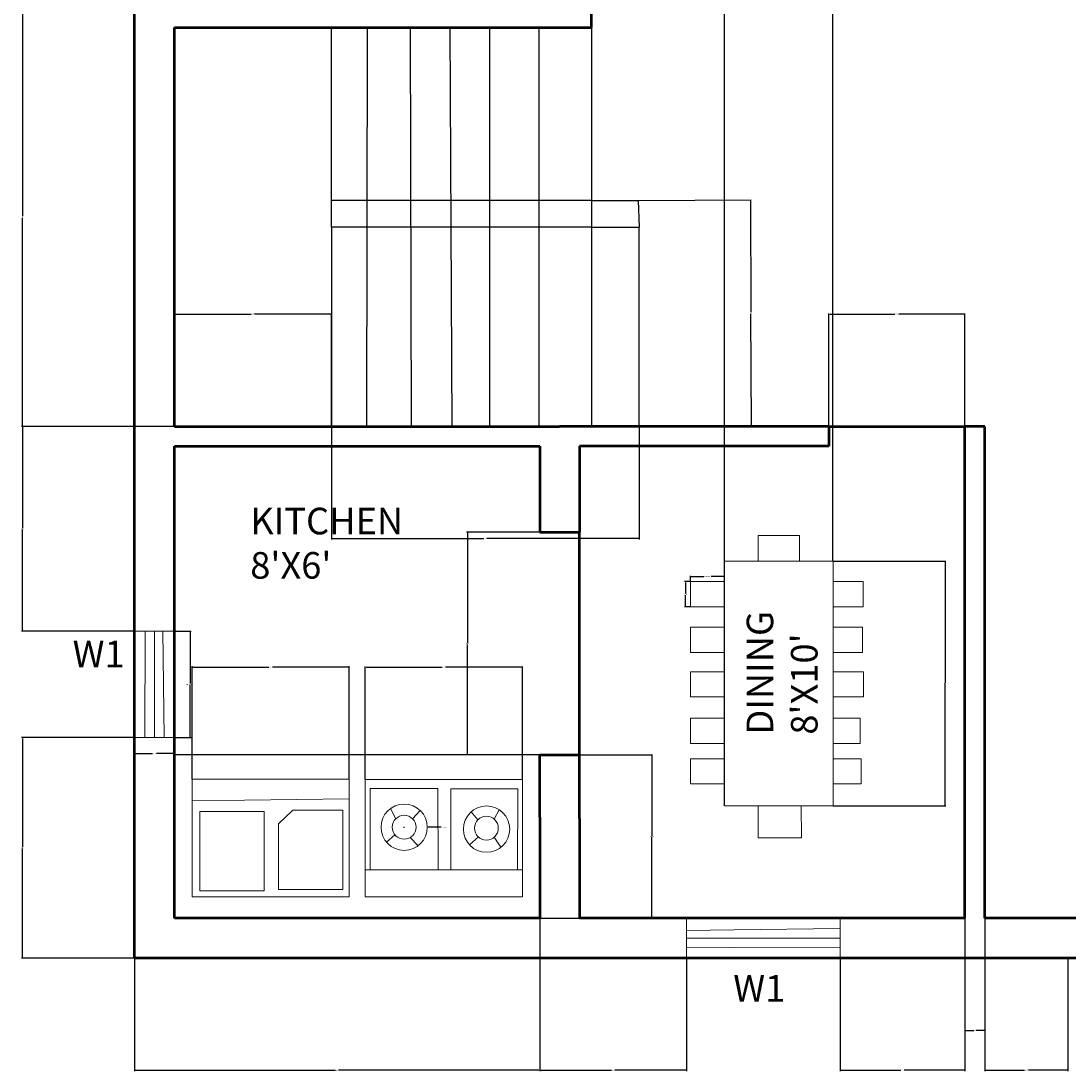
# Model space of a CAD drawing. Units: inches. Extents: x 2521 to 2933, y 1745 to 2276.
# Tile 1 of 4: x 2521 to 2758, y 1745 to 1982. Entities that reach past the tile are written whole.
import ezdxf

# ---------------------------------------------------------------- set-up
doc = ezdxf.new("R2010")
doc.units = ezdxf.units.IN
for name, color, linetype, lineweight in [('A-ANNO-DIMS', 2, 'Continuous', 18), ('A-ANNO-TEXT', 3, 'Continuous', 18), ('A-AREA-IDEN', 7, 'Continuous', 25), ('A-EQPM', 8, 'Continuous', 18), ('A-FLOR-CASE', 32, 'Continuous', 25), ('A-FLOR-FIXT', 9, 'Continuous', 18), ('A-FLOR-STRS', 7, 'Continuous', 25), ('A-FURN', 8, 'Continuous', 18), ('A-GLAZ', 4, 'Continuous', 20), ('A-WALL', 7, 'Continuous', 50)]:
    doc.layers.add(name, color=color, linetype=linetype, lineweight=lineweight)
doc.styles.get("Standard").update_dxf_attribs({"font": 'arial.ttf'})
doc.dimstyles.get("Standard").update_dxf_attribs({"dimtxt": 0.18, "dimasz": 0.18, "dimexe": 0.18, "dimexo": 0.0625, "dimgap": 0.09, "dimtad": 0, "dimtih": 1, "dimtoh": 1, "dimdec": 4, "dimzin": 0, "dimdsep": 46, "dimtxsty": 'Standard', "dimcen": 0.09, "dimadec": 0, "dimazin": 0, "dimtfac": 1, "dimtdec": 4, "dimtofl": 0, "dimtmove": 0, "dimatfit": 3, "dimfxl": 1, "dimtolj": 1, "dimtzin": 0, "dimarcsym": 0})

# ---------------------------------------------------------------- blocks, each defined once
blk = doc.blocks.new('WINDOW-W1-LONG')
for p, q in [((0, 24), (0, 34.69)), ((0, 34.69), (9, 34.69)), ((2.4, 24), (2.44, 34.69)), ((4.5, 24), (4.5, 34.69)), ((6.37, 24), (6.23, 34.69)), ((9, 34.69), (9, 24)), ((0, 24), (0, 0)), ((2.32, 0), (2.4, 24)), ((4.5, 0), (4.5, 24)), ((6.68, 0), (6.37, 24)), ((9, 24), (9, 0)), ((9, 0), (0, 0))]:
    blk.add_line(p, q)
blk = doc.blocks.new('WINDOW-24')
for p, q in [((9, 24), (0, 24)), ((0, 24), (0, 0)), ((2.32, 0), (2.4, 24)), ((4.5, 0), (4.5, 24)), ((6.68, 0), (6.37, 24)), ((9, 24), (9, 0)), ((9, 0), (0, 0))]:
    blk.add_line(p, q)
blk = doc.blocks.new('CHAIR-DINING-SIDE')
for p, q in [((0, 5.7), (7.67, 5.7)), ((0, 0), (0, 5.7)), ((7.67, 0), (0, 0))]:
    blk.add_line(p, q)
blk = doc.blocks.new('*D11')
at = {"layer": 'A-ANNO-DIMS', "color": 0, "lineweight": -2, "transparency": 16777216}
for p, q in [((2556.07, 1844.03), (2559.79, 1844.03)), ((2559.61, 1843.85), (2559.61, 1832.21)), ((2559.61, 1820.21), (2559.61, 1831.85)), ((2556.07, 1820.03), (2559.79, 1820.03))]:
    blk.add_line(p, q, dxfattribs=at)
at = {"layer": 'A-ANNO-DIMS', "color": 0, "transparency": 16777216}
for points in [[(2559.58, 1843.85), (2559.64, 1843.85), (2559.61, 1844.03)], [(2559.58, 1820.21), (2559.64, 1820.21), (2559.61, 1820.03)]]:
    blk.add_solid(points, dxfattribs=at)
at = {"layer": 'Defpoints', "color": 0, "transparency": 16777216}
for p in [(2556.01, 1844.03), (2559.61, 1844.03), (2556.01, 1820.03)]:
    blk.add_point(p, dxfattribs=at)
at = {"layer": 'A-ANNO-DIMS', "color": 0, "transparency": 16777216, "insert": (2559.61, 1832.03), "char_height": 0.18, "attachment_point": 5}
blk.add_mtext('\\A1;WINDOW 24 TYP.', dxfattribs=at)
blk = doc.blocks.new('*D12')
at = {"layer": 'A-ANNO-DIMS', "color": 0, "lineweight": -2, "transparency": 16777216}
for p, q in [((2547.01, 1819.97), (2547.01, 1816.25)), ((2556.01, 1819.97), (2556.01, 1816.25)), ((2547.19, 1816.43), (2551.05, 1816.43)), ((2555.83, 1816.43), (2551.97, 1816.43))]:
    blk.add_line(p, q, dxfattribs=at)
at = {"layer": 'A-ANNO-DIMS', "color": 0, "transparency": 16777216}
for points in [[(2547.19, 1816.46), (2547.19, 1816.4), (2547.01, 1816.43)], [(2555.83, 1816.46), (2555.83, 1816.4), (2556.01, 1816.43)]]:
    blk.add_solid(points, dxfattribs=at)
at = {"layer": 'Defpoints', "color": 0, "transparency": 16777216}
for p in [(2547.01, 1820.03), (2556.01, 1820.03), (2556.01, 1816.43)]:
    blk.add_point(p, dxfattribs=at)
at = {"layer": 'A-ANNO-DIMS', "color": 0, "transparency": 16777216, "insert": (2551.51, 1816.43), "char_height": 0.18, "attachment_point": 5}
blk.add_mtext('\\A1;9 TYP.', dxfattribs=at)
blk = doc.blocks.new('*D21')
at = {"layer": 'A-ANNO-DIMS', "color": 0, "lineweight": -2, "transparency": 16777216}
for p, q in [((2672.56, 1855.31), (2672.56, 1856.58)), ((2672.74, 1856.4), (2675.57, 1856.4)), ((2680.05, 1856.4), (2677.21, 1856.4)), ((2680.23, 1855.31), (2680.23, 1856.58))]:
    blk.add_line(p, q, dxfattribs=at)
at = {"layer": 'A-ANNO-DIMS', "color": 0, "transparency": 16777216}
for points in [[(2672.74, 1856.43), (2672.74, 1856.37), (2672.56, 1856.4)], [(2680.05, 1856.43), (2680.05, 1856.37), (2680.23, 1856.4)]]:
    blk.add_solid(points, dxfattribs=at)
at = {"layer": 'Defpoints', "color": 0, "transparency": 16777216}
for p in [(2680.23, 1856.4), (2672.56, 1855.25), (2680.23, 1855.25)]:
    blk.add_point(p, dxfattribs=at)
at = {"layer": 'A-ANNO-DIMS', "color": 0, "transparency": 16777216, "insert": (2676.39, 1856.4), "char_height": 0.18, "attachment_point": 5}
blk.add_mtext('\\A1;SEAT 8 TYP.', dxfattribs=at)
blk = doc.blocks.new('*D22')
at = {"layer": 'A-ANNO-DIMS', "color": 0, "lineweight": -2, "transparency": 16777216}
for p, q in [((2672.49, 1855.25), (2671.23, 1855.25)), ((2671.41, 1855.07), (2671.41, 1852.58)), ((2671.41, 1849.72), (2671.41, 1852.21)), ((2672.49, 1849.54), (2671.23, 1849.54))]:
    blk.add_line(p, q, dxfattribs=at)
at = {"layer": 'A-ANNO-DIMS', "color": 0, "transparency": 16777216}
for points in [[(2671.38, 1855.07), (2671.44, 1855.07), (2671.41, 1855.25)], [(2671.38, 1849.72), (2671.44, 1849.72), (2671.41, 1849.54)]]:
    blk.add_solid(points, dxfattribs=at)
at = {"layer": 'Defpoints', "color": 0, "transparency": 16777216}
for p in [(2671.41, 1855.25), (2672.56, 1855.25), (2672.56, 1849.54)]:
    blk.add_point(p, dxfattribs=at)
at = {"layer": 'A-ANNO-DIMS', "color": 0, "transparency": 16777216, "insert": (2671.41, 1852.4), "char_height": 0.18, "attachment_point": 5}
blk.add_mtext('\\A1;6 TYP.', dxfattribs=at)
blk = doc.blocks.new('*D29')
at = {"layer": 'A-ANNO-DIMS', "color": 0, "lineweight": -2, "transparency": 16777216}
for p, q in [((2546.95, 1820.03), (2521.51, 1820.03)), ((2521.69, 1819.85), (2521.69, 1795.34)), ((2521.69, 1770.46), (2521.69, 1794.97)), ((2546.95, 1770.28), (2521.51, 1770.28))]:
    blk.add_line(p, q, dxfattribs=at)
at = {"layer": 'A-ANNO-DIMS', "color": 0, "transparency": 16777216}
for points in [[(2521.66, 1819.85), (2521.72, 1819.85), (2521.69, 1820.03)], [(2521.66, 1770.46), (2521.72, 1770.46), (2521.69, 1770.28)]]:
    blk.add_solid(points, dxfattribs=at)
at = {"layer": 'Defpoints', "color": 0, "transparency": 16777216}
for p in [(2521.69, 1820.03), (2547.01, 1820.03), (2547.01, 1770.28)]:
    blk.add_point(p, dxfattribs=at)
at = {"layer": 'A-ANNO-DIMS', "color": 0, "transparency": 16777216, "insert": (2521.69, 1795.16), "char_height": 0.18, "attachment_point": 5}
blk.add_mtext('\\A1;49.75', dxfattribs=at)
blk = doc.blocks.new('*D30')
at = {"layer": 'A-ANNO-DIMS', "color": 0, "lineweight": -2, "transparency": 16777216}
for p, q in [((2555.95, 1890.28), (2521.51, 1890.28)), ((2521.69, 1890.1), (2521.69, 1867.34)), ((2521.69, 1844.21), (2521.69, 1866.97)), ((2546.95, 1844.03), (2521.51, 1844.03))]:
    blk.add_line(p, q, dxfattribs=at)
at = {"layer": 'A-ANNO-DIMS', "color": 0, "transparency": 16777216}
for points in [[(2521.66, 1890.1), (2521.72, 1890.1), (2521.69, 1890.28)], [(2521.66, 1844.21), (2521.72, 1844.21), (2521.69, 1844.03)]]:
    blk.add_solid(points, dxfattribs=at)
at = {"layer": 'Defpoints', "color": 0, "transparency": 16777216}
for p in [(2521.69, 1890.28), (2556.01, 1890.28), (2547.01, 1844.03)]:
    blk.add_point(p, dxfattribs=at)
at = {"layer": 'A-ANNO-DIMS', "color": 0, "transparency": 16777216, "insert": (2521.69, 1867.16), "char_height": 0.18, "attachment_point": 5}
blk.add_mtext('\\A1;46.25', dxfattribs=at)
blk = doc.blocks.new('*D31')
at = {"layer": 'A-ANNO-DIMS', "color": 0, "lineweight": -2, "transparency": 16777216}
for p, q in [((2555.95, 1984.78), (2521.51, 1984.78)), ((2521.69, 1984.6), (2521.69, 1937.71)), ((2521.69, 1890.46), (2521.69, 1937.35)), ((2555.95, 1890.28), (2521.51, 1890.28))]:
    blk.add_line(p, q, dxfattribs=at)
at = {"layer": 'A-ANNO-DIMS', "color": 0, "transparency": 16777216}
for points in [[(2521.66, 1984.6), (2521.72, 1984.6), (2521.69, 1984.78)], [(2521.66, 1890.46), (2521.72, 1890.46), (2521.69, 1890.28)]]:
    blk.add_solid(points, dxfattribs=at)
at = {"layer": 'Defpoints', "color": 0, "transparency": 16777216}
for p in [(2521.69, 1984.78), (2556.01, 1984.78), (2556.01, 1890.28)]:
    blk.add_point(p, dxfattribs=at)
at = {"layer": 'A-ANNO-DIMS', "color": 0, "transparency": 16777216, "insert": (2521.69, 1937.53), "char_height": 0.18, "attachment_point": 5}
blk.add_mtext('\\A1;94.5', dxfattribs=at)
blk = doc.blocks.new('*D39')
at = {"layer": 'A-ANNO-DIMS', "color": 0, "lineweight": -2, "transparency": 16777216}
for p, q in [((2638.51, 1779.22), (2638.51, 1744.78)), ((2547.01, 1770.22), (2547.01, 1744.78)), ((2547.19, 1744.96), (2592.43, 1744.96)), ((2638.33, 1744.96), (2593.08, 1744.96))]:
    blk.add_line(p, q, dxfattribs=at)
at = {"layer": 'A-ANNO-DIMS', "color": 0, "transparency": 16777216}
for points in [[(2547.19, 1744.99), (2547.19, 1744.93), (2547.01, 1744.96)], [(2638.33, 1744.99), (2638.33, 1744.93), (2638.51, 1744.96)]]:
    blk.add_solid(points, dxfattribs=at)
at = {"layer": 'Defpoints', "color": 0, "transparency": 16777216}
for p in [(2638.51, 1779.28), (2547.01, 1770.28), (2638.51, 1744.96)]:
    blk.add_point(p, dxfattribs=at)
at = {"layer": 'A-ANNO-DIMS', "color": 0, "transparency": 16777216, "insert": (2592.76, 1744.96), "char_height": 0.18, "attachment_point": 5}
blk.add_mtext('\\A1;91.5', dxfattribs=at)
blk = doc.blocks.new('*D40')
at = {"layer": 'A-ANNO-DIMS', "color": 0, "lineweight": -2, "transparency": 16777216}
for p, q in [((2638.51, 1779.22), (2638.51, 1744.78)), ((2671.68, 1770.22), (2671.68, 1744.78)), ((2638.69, 1744.96), (2654.7, 1744.96)), ((2671.5, 1744.96), (2655.49, 1744.96))]:
    blk.add_line(p, q, dxfattribs=at)
at = {"layer": 'A-ANNO-DIMS', "color": 0, "transparency": 16777216}
for points in [[(2638.69, 1744.99), (2638.69, 1744.93), (2638.51, 1744.96)], [(2671.5, 1744.99), (2671.5, 1744.93), (2671.68, 1744.96)]]:
    blk.add_solid(points, dxfattribs=at)
at = {"layer": 'Defpoints', "color": 0, "transparency": 16777216}
for p in [(2638.51, 1779.28), (2671.68, 1770.28), (2671.68, 1744.96)]:
    blk.add_point(p, dxfattribs=at)
at = {"layer": 'A-ANNO-DIMS', "color": 0, "transparency": 16777216, "insert": (2655.09, 1744.96), "char_height": 0.18, "attachment_point": 5}
blk.add_mtext('\\A1;33.17', dxfattribs=at)
blk = doc.blocks.new('*D41')
at = {"layer": 'A-ANNO-DIMS', "color": 0, "lineweight": -2, "transparency": 16777216}
for p, q in [((2734.51, 1779.22), (2734.51, 1744.78)), ((2706.37, 1770.22), (2706.37, 1744.78)), ((2706.55, 1744.96), (2720.05, 1744.96)), ((2734.33, 1744.96), (2720.83, 1744.96))]:
    blk.add_line(p, q, dxfattribs=at)
at = {"layer": 'A-ANNO-DIMS', "color": 0, "transparency": 16777216}
for points in [[(2706.55, 1744.99), (2706.55, 1744.93), (2706.37, 1744.96)], [(2734.33, 1744.99), (2734.33, 1744.93), (2734.51, 1744.96)]]:
    blk.add_solid(points, dxfattribs=at)
at = {"layer": 'Defpoints', "color": 0, "transparency": 16777216}
for p in [(2734.51, 1779.28), (2706.37, 1770.28), (2734.51, 1744.96)]:
    blk.add_point(p, dxfattribs=at)
at = {"layer": 'A-ANNO-DIMS', "color": 0, "transparency": 16777216, "insert": (2720.44, 1744.96), "char_height": 0.18, "attachment_point": 5}
blk.add_mtext('\\A1;28.14', dxfattribs=at)
blk = doc.blocks.new('*D42')
at = {"layer": 'A-ANNO-DIMS', "color": 0, "lineweight": -2, "transparency": 16777216}
for p, q in [((2734.51, 1779.22), (2734.51, 1753.78)), ((2739.01, 1779.22), (2739.01, 1753.78)), ((2734.69, 1753.96), (2736.5, 1753.96)), ((2738.83, 1753.96), (2737.02, 1753.96))]:
    blk.add_line(p, q, dxfattribs=at)
at = {"layer": 'A-ANNO-DIMS', "color": 0, "transparency": 16777216}
for points in [[(2734.69, 1753.99), (2734.69, 1753.93), (2734.51, 1753.96)], [(2738.83, 1753.99), (2738.83, 1753.93), (2739.01, 1753.96)]]:
    blk.add_solid(points, dxfattribs=at)
at = {"layer": 'Defpoints', "color": 0, "transparency": 16777216}
for p in [(2734.51, 1779.28), (2739.01, 1779.28), (2734.51, 1753.96)]:
    blk.add_point(p, dxfattribs=at)
at = {"layer": 'A-ANNO-DIMS', "color": 0, "transparency": 16777216, "insert": (2736.76, 1753.96), "char_height": 0.18, "attachment_point": 5}
blk.add_mtext('\\A1;4.5', dxfattribs=at)
blk = doc.blocks.new('*D43')
at = {"layer": 'A-ANNO-DIMS', "color": 0, "lineweight": -2, "transparency": 16777216}
for p, q in [((2739.01, 1779.22), (2739.01, 1744.78)), ((2757.79, 1770.22), (2757.79, 1744.78)), ((2739.19, 1744.96), (2747.95, 1744.96)), ((2757.61, 1744.96), (2748.86, 1744.96))]:
    blk.add_line(p, q, dxfattribs=at)
at = {"layer": 'A-ANNO-DIMS', "color": 0, "transparency": 16777216}
for points in [[(2739.19, 1744.99), (2739.19, 1744.93), (2739.01, 1744.96)], [(2757.61, 1744.99), (2757.61, 1744.93), (2757.79, 1744.96)]]:
    blk.add_solid(points, dxfattribs=at)
at = {"layer": 'Defpoints', "color": 0, "transparency": 16777216}
for p in [(2739.01, 1779.28), (2757.79, 1770.28), (2757.79, 1744.96)]:
    blk.add_point(p, dxfattribs=at)
at = {"layer": 'A-ANNO-DIMS', "color": 0, "transparency": 16777216, "insert": (2748.4, 1744.96), "char_height": 0.18, "attachment_point": 5}
blk.add_mtext('\\A1;18.785', dxfattribs=at)
blk = doc.blocks.new('*D45')
at = {"layer": 'A-ANNO-DIMS', "color": 0, "lineweight": -2, "transparency": 16777216}
for p, q in [((2556.01, 1890.34), (2556.01, 1915.78)), ((2556.19, 1915.6), (2573.35, 1915.6)), ((2591.3, 1915.6), (2574.14, 1915.6)), ((2591.48, 1890.34), (2591.48, 1915.78))]:
    blk.add_line(p, q, dxfattribs=at)
at = {"layer": 'A-ANNO-DIMS', "color": 0, "transparency": 16777216}
for points in [[(2556.19, 1915.63), (2556.19, 1915.57), (2556.01, 1915.6)], [(2591.3, 1915.63), (2591.3, 1915.57), (2591.48, 1915.6)]]:
    blk.add_solid(points, dxfattribs=at)
at = {"layer": 'Defpoints', "color": 0, "transparency": 16777216}
for p in [(2591.48, 1915.6), (2556.01, 1890.28), (2591.48, 1890.28)]:
    blk.add_point(p, dxfattribs=at)
at = {"layer": 'A-ANNO-DIMS', "color": 0, "transparency": 16777216, "insert": (2573.75, 1915.6), "char_height": 0.18, "attachment_point": 5}
blk.add_mtext('\\A1;35.47', dxfattribs=at)
blk = doc.blocks.new('*D46')
at = {"layer": 'A-ANNO-DIMS', "color": 0, "lineweight": -2, "transparency": 16777216}
for p, q in [((2591.48, 1890.22), (2591.48, 1864.78)), ((2660.98, 1890.22), (2660.98, 1864.78)), ((2591.66, 1864.96), (2625.91, 1864.96)), ((2660.8, 1864.96), (2626.56, 1864.96))]:
    blk.add_line(p, q, dxfattribs=at)
at = {"layer": 'A-ANNO-DIMS', "color": 0, "transparency": 16777216}
for points in [[(2591.66, 1864.99), (2591.66, 1864.93), (2591.48, 1864.96)], [(2660.8, 1864.99), (2660.8, 1864.93), (2660.98, 1864.96)]]:
    blk.add_solid(points, dxfattribs=at)
at = {"layer": 'Defpoints', "color": 0, "transparency": 16777216}
for p in [(2591.48, 1890.28), (2660.98, 1890.28), (2591.48, 1864.96)]:
    blk.add_point(p, dxfattribs=at)
at = {"layer": 'A-ANNO-DIMS', "color": 0, "transparency": 16777216, "insert": (2626.23, 1864.96), "char_height": 0.18, "attachment_point": 5}
blk.add_mtext('\\A1;69.5', dxfattribs=at)
blk = doc.blocks.new('*D47')
at = {"layer": 'A-ANNO-DIMS', "color": 0, "lineweight": -2, "transparency": 16777216}
for p, q in [((2660.82, 1941.28), (2686.26, 1941.39)), ((2686.08, 1941.21), (2686.19, 1916.07)), ((2686.3, 1890.57), (2686.19, 1915.71)), ((2661.05, 1890.28), (2686.48, 1890.39))]:
    blk.add_line(p, q, dxfattribs=at)
at = {"layer": 'A-ANNO-DIMS', "color": 0, "transparency": 16777216}
for points in [[(2686.11, 1941.21), (2686.05, 1941.21), (2686.08, 1941.39)], [(2686.33, 1890.57), (2686.27, 1890.57), (2686.3, 1890.39)]]:
    blk.add_solid(points, dxfattribs=at)
at = {"layer": 'Defpoints', "color": 0, "transparency": 16777216}
for p in [(2660.76, 1941.28), (2660.98, 1890.28), (2686.3, 1890.39)]:
    blk.add_point(p, dxfattribs=at)
at = {"layer": 'A-ANNO-DIMS', "color": 0, "transparency": 16777216, "insert": (2686.19, 1915.89), "char_height": 0.18, "attachment_point": 5}
blk.add_mtext('\\A1;51', dxfattribs=at)
blk = doc.blocks.new('*D50')
at = {"layer": 'A-ANNO-DIMS', "color": 0, "lineweight": -2, "transparency": 16777216}
for p, q in [((2647.45, 1866.41), (2622.01, 1866.4)), ((2622.19, 1866.22), (2622.2, 1841.45)), ((2622.21, 1816.31), (2622.2, 1841.08)), ((2647.46, 1816.14), (2622.03, 1816.13))]:
    blk.add_line(p, q, dxfattribs=at)
at = {"layer": 'A-ANNO-DIMS', "color": 0, "transparency": 16777216}
for points in [[(2622.22, 1866.22), (2622.16, 1866.22), (2622.19, 1866.4)], [(2622.24, 1816.31), (2622.18, 1816.31), (2622.21, 1816.13)]]:
    blk.add_solid(points, dxfattribs=at)
at = {"layer": 'Defpoints', "color": 0, "transparency": 16777216}
for p in [(2622.19, 1866.4), (2647.51, 1866.41), (2647.53, 1816.14)]:
    blk.add_point(p, dxfattribs=at)
at = {"layer": 'A-ANNO-DIMS', "color": 0, "transparency": 16777216, "insert": (2622.2, 1841.27), "char_height": 0.18, "attachment_point": 5}
blk.add_mtext('\\A1;50.27', dxfattribs=at)
blk = doc.blocks.new('*D51')
at = {"layer": 'A-ANNO-DIMS', "color": 0, "lineweight": -2, "transparency": 16777216}
for p, q in [((2703.8, 1890.34), (2703.8, 1915.78)), ((2703.98, 1915.6), (2718.7, 1915.6)), ((2734.35, 1915.6), (2719.63, 1915.6)), ((2734.53, 1890.34), (2734.53, 1915.78))]:
    blk.add_line(p, q, dxfattribs=at)
at = {"layer": 'A-ANNO-DIMS', "color": 0, "transparency": 16777216}
for points in [[(2703.98, 1915.63), (2703.98, 1915.57), (2703.8, 1915.6)], [(2734.35, 1915.63), (2734.35, 1915.57), (2734.53, 1915.6)]]:
    blk.add_solid(points, dxfattribs=at)
at = {"layer": 'Defpoints', "color": 0, "transparency": 16777216}
for p in [(2734.53, 1915.6), (2703.8, 1890.28), (2734.53, 1890.28)]:
    blk.add_point(p, dxfattribs=at)
at = {"layer": 'A-ANNO-DIMS', "color": 0, "transparency": 16777216, "insert": (2719.16, 1915.6), "char_height": 0.18, "attachment_point": 5}
blk.add_mtext('\\A1;30.734', dxfattribs=at)
blk = doc.blocks.new('*D52')
at = {"layer": 'A-ANNO-DIMS', "color": 0, "lineweight": -2, "transparency": 16777216}
for p, q in [((2638.57, 1816.14), (2664.01, 1816.14)), ((2663.83, 1815.96), (2663.83, 1797.89)), ((2663.83, 1779.46), (2663.83, 1797.53)), ((2638.57, 1779.28), (2664.01, 1779.28))]:
    blk.add_line(p, q, dxfattribs=at)
at = {"layer": 'A-ANNO-DIMS', "color": 0, "transparency": 16777216}
for points in [[(2663.8, 1815.96), (2663.86, 1815.96), (2663.83, 1816.14)], [(2663.8, 1779.46), (2663.86, 1779.46), (2663.83, 1779.28)]]:
    blk.add_solid(points, dxfattribs=at)
at = {"layer": 'Defpoints', "color": 0, "transparency": 16777216}
for p in [(2638.51, 1816.14), (2638.51, 1779.28), (2663.83, 1779.28)]:
    blk.add_point(p, dxfattribs=at)
at = {"layer": 'A-ANNO-DIMS', "color": 0, "transparency": 16777216, "insert": (2663.83, 1797.71), "char_height": 0.18, "attachment_point": 5}
blk.add_mtext('\\A1;36.856', dxfattribs=at)
blk = doc.blocks.new('*D53')
at = {"layer": 'A-ANNO-DIMS', "color": 0, "lineweight": -2, "transparency": 16777216}
for p, q in [((2560.04, 1810.69), (2560.04, 1836.13)), ((2560.22, 1835.95), (2577.38, 1835.95)), ((2595.33, 1835.95), (2578.17, 1835.95)), ((2595.51, 1810.69), (2595.51, 1836.13))]:
    blk.add_line(p, q, dxfattribs=at)
at = {"layer": 'A-ANNO-DIMS', "color": 0, "transparency": 16777216}
for points in [[(2560.22, 1835.98), (2560.22, 1835.92), (2560.04, 1835.95)], [(2595.33, 1835.98), (2595.33, 1835.92), (2595.51, 1835.95)]]:
    blk.add_solid(points, dxfattribs=at)
at = {"layer": 'Defpoints', "color": 0, "transparency": 16777216}
for p in [(2595.51, 1835.95), (2560.04, 1810.63), (2595.51, 1810.63)]:
    blk.add_point(p, dxfattribs=at)
at = {"layer": 'A-ANNO-DIMS', "color": 0, "transparency": 16777216, "insert": (2577.78, 1835.95), "char_height": 0.18, "attachment_point": 5}
blk.add_mtext('\\A1;35.47', dxfattribs=at)
blk = doc.blocks.new('*D54')
at = {"layer": 'A-ANNO-DIMS', "color": 0, "lineweight": -2, "transparency": 16777216}
for p, q in [((2599.13, 1810.65), (2599.13, 1836.09)), ((2599.31, 1835.91), (2616.47, 1835.91)), ((2634.42, 1835.91), (2617.26, 1835.91)), ((2634.6, 1810.65), (2634.6, 1836.09))]:
    blk.add_line(p, q, dxfattribs=at)
at = {"layer": 'A-ANNO-DIMS', "color": 0, "transparency": 16777216}
for points in [[(2599.31, 1835.94), (2599.31, 1835.88), (2599.13, 1835.91)], [(2634.42, 1835.94), (2634.42, 1835.88), (2634.6, 1835.91)]]:
    blk.add_solid(points, dxfattribs=at)
at = {"layer": 'Defpoints', "color": 0, "transparency": 16777216}
for p in [(2634.6, 1835.91), (2599.13, 1810.59), (2634.6, 1810.59)]:
    blk.add_point(p, dxfattribs=at)
at = {"layer": 'A-ANNO-DIMS', "color": 0, "transparency": 16777216, "insert": (2616.86, 1835.91), "char_height": 0.18, "attachment_point": 5}
blk.add_mtext('\\A1;35.47', dxfattribs=at)
blk = doc.blocks.new('*D55')
at = {"layer": 'A-ANNO-DIMS', "color": 0, "lineweight": -2, "transparency": 16777216}
for p, q in [((2680.23, 1804.66), (2680.23, 2275.78)), ((2680.41, 2275.6), (2692.15, 2275.6)), ((2704.55, 2275.6), (2692.81, 2275.6)), ((2704.73, 1859.95), (2704.73, 2275.78))]:
    blk.add_line(p, q, dxfattribs=at)
at = {"layer": 'A-ANNO-DIMS', "color": 0, "transparency": 16777216}
for points in [[(2680.41, 2275.63), (2680.41, 2275.57), (2680.23, 2275.6)], [(2704.55, 2275.63), (2704.55, 2275.57), (2704.73, 2275.6)]]:
    blk.add_solid(points, dxfattribs=at)
at = {"layer": 'Defpoints', "color": 0, "transparency": 16777216}
for p in [(2704.73, 2275.6), (2704.73, 1859.89), (2680.23, 1804.6)]:
    blk.add_point(p, dxfattribs=at)
at = {"layer": 'A-ANNO-DIMS', "color": 0, "transparency": 16777216, "insert": (2692.48, 2275.6), "char_height": 0.18, "attachment_point": 5}
blk.add_mtext('\\A1;24.5', dxfattribs=at)
blk = doc.blocks.new('*D56')
at = {"layer": 'A-ANNO-DIMS', "color": 0, "lineweight": -2, "transparency": 16777216}
for p, q in [((2704.79, 1859.89), (2730.23, 1859.89)), ((2730.05, 1859.71), (2730.05, 1832.43)), ((2730.05, 1804.78), (2730.05, 1832.06)), ((2704.79, 1804.6), (2730.23, 1804.6))]:
    blk.add_line(p, q, dxfattribs=at)
at = {"layer": 'A-ANNO-DIMS', "color": 0, "transparency": 16777216}
for points in [[(2730.02, 1859.71), (2730.08, 1859.71), (2730.05, 1859.89)], [(2730.02, 1804.78), (2730.08, 1804.78), (2730.05, 1804.6)]]:
    blk.add_solid(points, dxfattribs=at)
at = {"layer": 'Defpoints', "color": 0, "transparency": 16777216}
for p in [(2704.73, 1859.89), (2704.73, 1804.6), (2730.05, 1804.6)]:
    blk.add_point(p, dxfattribs=at)
at = {"layer": 'A-ANNO-DIMS', "color": 0, "transparency": 16777216, "insert": (2730.05, 1832.24), "char_height": 0.18, "attachment_point": 5}
blk.add_mtext('\\A1;55.3', dxfattribs=at)
blk = doc.blocks.new('*D66')
at = {"layer": 'A-ANNO-DIMS', "color": 0, "lineweight": -2, "transparency": 16777216}
for p, q in [((2607.81, 1799.8), (2607.99, 1799.8)), ((2607.9, 1799.71), (2607.9, 1799.89)), ((2616.26, 1799.8), (2613.31, 1799.8))]:
    blk.add_line(p, q, dxfattribs=at)
at = {"layer": 'A-ANNO-DIMS', "color": 0, "transparency": 16777216}
blk.add_solid([(2613.31, 1799.83), (2613.31, 1799.77), (2613.13, 1799.8)], dxfattribs=at)
at = {"layer": 'Defpoints', "color": 0, "transparency": 16777216}
for p in [(2602.68, 1799.8), (2613.13, 1799.8)]:
    blk.add_point(p, dxfattribs=at)
at = {"layer": 'A-ANNO-DIMS', "color": 0, "transparency": 16777216, "insert": (2616.94, 1799.8), "char_height": 0.18, "attachment_point": 5}
blk.add_mtext('\\A1;2X ∅10.45', dxfattribs=at)

msp = doc.modelspace()

# ---------------------------------------------------------------- linework, layer by layer
at = {"layer": 'A-EQPM'}
for p, q in [((2600.2102, 1790.1554), (2600.2102, 1808.5242)), ((2600.2102, 1808.5242), (2615.4727, 1808.5242)), ((2615.4727, 1808.5242), (2615.6004, 1790.1554)), ((2618.4102, 1790.1554), (2618.4102, 1808.4604)), ((2618.4102, 1808.4604), (2633.545, 1808.4604)), ((2633.545, 1808.4604), (2633.4811, 1790.1554)), ((2606.0085, 1801.7142), (2604.8169, 1804.0179)), ((2609.788, 1801.7183), (2611.479, 1803.6067)), ((2628.257, 1801.5979), (2629.3835, 1803.7275)), ((2624.5099, 1801.4415), (2623.0559, 1803.3017)), ((2605.8226, 1798.0892), (2603.924, 1796.4107)), ((2609.263, 1797.4791), (2611.0454, 1795.6278)), ((2624.652, 1797.6008), (2622.6313, 1795.8582)), ((2628.1942, 1797.5293), (2629.7429, 1795.2761)), ((2599.1296, 1790.1554), (2634.5962, 1790.1554))]:
    msp.add_line(p, q, dxfattribs=at)
msp.add_lwpolyline([(2599.1296, 1810.5872), (2634.5962, 1810.5872), (2634.5962, 1784.0733), (2599.1296, 1784.0733)], close=True, dxfattribs=at)
for centre, radius in [((2607.9003, 1799.8), 5.2248), ((2626.4985, 1799.3715), 5.2248), ((2607.9003, 1799.8), 2.6914), ((2626.4639, 1799.5908), 2.6914)]:
    msp.add_circle(centre, radius, dxfattribs=at)
at = {"layer": 'A-FLOR-CASE'}
msp.add_line((2638.509, 1816.1379), (2556.009, 1816.1379), dxfattribs=at)
at = {"layer": 'A-FLOR-FIXT'}
for p, q in [((2560.0418, 1805.7514), (2595.5085, 1806.2387)), ((2579.4926, 1800.6066), (2582.7822, 1803.6651))]:
    msp.add_line(p, q, dxfattribs=at)
for points in [[(2560.0418, 1810.6258), (2595.5085, 1810.6258), (2595.5085, 1784.1118), (2560.0418, 1784.1118)], [(2561.7802, 1803.3582), (2576.3187, 1803.3582), (2576.3187, 1785.456), (2561.7802, 1785.456)]]:
    msp.add_lwpolyline(points, close=True, dxfattribs=at)
msp.add_lwpolyline([(2582.7822, 1803.6651), (2594.0312, 1803.6651), (2594.0312, 1785.7629), (2579.4926, 1785.7629), (2579.4926, 1800.6066)], dxfattribs=at)
at = {"layer": 'A-FLOR-STRS'}
for p, q in [((2591.4825, 1935.2819), (2591.4825, 1980.2819)), ((2599.509, 1890.2819), (2599.6108, 1980.2819)), ((2609.5475, 1890.2819), (2609.3527, 1980.2819)), ((2618.7048, 1890.2819), (2618.3152, 1980.2819)), ((2627.2776, 1890.2819), (2627.2776, 1980.2819)), ((2638.3833, 1890.2819), (2638.3833, 1980.2819)), ((2650.1821, 1980.2819), (2650.1985, 1890.2819)), ((2650.1903, 1941.2819), (2591.4825, 1941.2819)), ((2650.1892, 1941.2819), (2660.7615, 1941.2819)), ((2660.7615, 1941.2819), (2660.9844, 1935.2819)), ((2650.1903, 1935.2819), (2591.4825, 1935.2819)), ((2591.4825, 1935.2819), (2591.4825, 1890.2819)), ((2650.1903, 1935.2819), (2660.9844, 1935.2819)), ((2660.9844, 1890.2819), (2660.9844, 1935.2819))]:
    msp.add_line(p, q, dxfattribs=at)
at = {"layer": 'A-FURN'}
for p, q in [((2687.8509, 1859.892), (2687.8509, 1865.6547)), ((2687.8509, 1865.6547), (2697.1471, 1865.6547)), ((2697.1471, 1865.6547), (2697.1471, 1859.892)), ((2704.7306, 1855.2473), (2710.8122, 1855.2473)), ((2710.8122, 1855.2473), (2711.552, 1855.2473)), ((2711.552, 1855.2473), (2711.552, 1849.5427)), ((2710.8122, 1849.5439), (2704.7306, 1849.5439)), ((2710.8122, 1849.5439), (2711.552, 1849.5427)), ((2704.7306, 1844.9748), (2710.664, 1844.9748)), ((2710.664, 1844.9748), (2711.4038, 1844.9748)), ((2711.4038, 1844.9748), (2711.4038, 1839.2703)), ((2710.664, 1839.2715), (2704.7306, 1839.2715)), ((2710.664, 1839.2715), (2711.4038, 1839.2703)), ((2704.7306, 1834.9169), (2710.8871, 1834.9169)), ((2710.8871, 1834.9169), (2711.6268, 1834.9169)), ((2711.6268, 1834.9169), (2711.6268, 1829.2123)), ((2710.8871, 1829.2135), (2704.7306, 1829.2135)), ((2710.8871, 1829.2135), (2711.6268, 1829.2123)), ((2704.7306, 1824.4399), (2710.1063, 1824.4399)), ((2710.1063, 1824.4399), (2710.846, 1824.4399)), ((2710.846, 1824.4399), (2710.846, 1818.7353)), ((2710.1063, 1818.7365), (2704.7306, 1818.7365)), ((2710.1063, 1818.7365), (2710.846, 1818.7353)), ((2704.7306, 1815.2789), (2710.3294, 1815.2789)), ((2710.3294, 1815.2789), (2711.0691, 1815.2789)), ((2711.0691, 1815.2789), (2711.0691, 1809.5743)), ((2710.3294, 1809.5755), (2704.7306, 1809.5755)), ((2710.3294, 1809.5755), (2711.0691, 1809.5743)), ((2687.8509, 1804.5971), (2687.8509, 1797.4466)), ((2697.6346, 1797.4466), (2697.5788, 1804.5971)), ((2687.8509, 1797.4466), (2697.6346, 1797.4466))]:
    msp.add_line(p, q, dxfattribs=at)
msp.add_lwpolyline([(2680.2296, 1859.892), (2704.7306, 1859.892), (2704.7306, 1804.5971), (2680.2296, 1804.5971)], close=True, dxfattribs=at)
at = {"layer": 'A-WALL'}
for p, q in [((2547.009, 1770.2819), (2547.009, 2250.2819)), ((2650.1821, 1980.2819), (2650.1821, 1984.7819)), ((2556.009, 1980.2819), (2628.009, 1980.2819)), ((2556.009, 1890.2819), (2556.009, 1980.2819)), ((2628.009, 1980.2819), (2650.1821, 1980.2819)), ((2556.009, 1890.2819), (2643.009, 1890.2819)), ((2703.7954, 1890.2819), (2643.009, 1890.2819)), ((2703.7954, 1890.2819), (2703.7954, 1885.7819)), ((2703.7954, 1890.2819), (2734.5297, 1890.2819)), ((2734.509, 1885.7819), (2734.5297, 1890.2819)), ((2739.009, 1890.2819), (2734.5297, 1890.2819)), ((2739.009, 1779.2819), (2739.009, 1890.2819)), ((2556.009, 1779.2819), (2556.009, 1885.7819)), ((2556.009, 1885.7819), (2638.509, 1885.7819)), ((2638.509, 1885.7819), (2638.509, 1866.4104)), ((2703.7954, 1885.7819), (2647.509, 1885.7819)), ((2647.509, 1885.7819), (2647.509, 1866.4104)), ((2734.509, 1779.2819), (2734.509, 1885.7819)), ((2638.509, 1866.4104), (2647.509, 1866.4104)), ((2647.5252, 1816.1379), (2647.509, 1866.4104)), ((2638.509, 1802.0453), (2638.509, 1816.1379)), ((2638.509, 1816.1379), (2647.5252, 1816.1379)), ((2647.509, 1801.7988), (2647.5252, 1816.1379)), ((2638.509, 1802.0453), (2638.509, 1779.2819)), ((2647.509, 1801.7988), (2647.509, 1779.2819)), ((2638.509, 1779.2819), (2556.009, 1779.2819)), ((2734.509, 1779.2819), (2647.509, 1779.2819)), ((2843.3859, 1779.2819), (2739.009, 1779.2819)), ((2843.4686, 1770.2819), (2547.009, 1770.2819))]:
    msp.add_line(p, q, dxfattribs=at)

# ---------------------------------------------------------------- block references
at = {"layer": 'A-FURN'}
for p in [(2672.557, 1849.544), (2672.557, 1839.2716), (2672.557, 1829.2136), (2672.557, 1818.7366), (2672.557, 1809.5756)]:
    msp.add_blockref('CHAIR-DINING-SIDE', p, dxfattribs=at)
at = {"layer": 'A-GLAZ'}
msp.add_blockref('WINDOW-24', (2547.009, 1820.032), dxfattribs=at)
at = {"layer": 'A-GLAZ', "rotation": 89.99999999999973}
msp.add_blockref('WINDOW-W1-LONG', (2706.3711, 1770.2819), dxfattribs=at)

# ---------------------------------------------------------------- texts
at = {"layer": 'A-ANNO-TEXT', "char_height": 6, "attachment_point": 1}
for width, insert in [(9.349954, (2533.0441, 1841.904)), (14.604376, (2682.2058, 1766.4486))]:
    msp.add_mtext_dynamic_manual_height_columns('W1', width=width, gutter_width=5.8967, heights=[0], dxfattribs=dict(at, insert=insert))
at = {"layer": 'A-AREA-IDEN', "insert": (2573.1511, 1871.9156), "char_height": 6, "attachment_point": 1}
msp.add_mtext_dynamic_manual_height_columns("KITCHEN \\P8'X6'", width=52.785185, gutter_width=5.8967, heights=[0], dxfattribs=at)
at = {"layer": 'A-AREA-IDEN', "insert": (2685.2348, 1820.6974), "char_height": 6, "attachment_point": 1, "rotation": 90}
msp.add_mtext_dynamic_manual_height_columns("DINING\\P8'X10'", width=5.248854, gutter_width=5.8967, heights=[0], dxfattribs=at)

# ---------------------------------------------------------------- dimensions: what is measured, and where the dimension line sits
at = {"layer": 'A-ANNO-DIMS'}
for base, p1, p2, override, picture, middle in [((2704.7306, 2275.6019), (2680.2296, 1804.5971), (2704.7306, 1859.892), {"dimdec": 1, "dimlfac": 1, "dimrnd": 0, "dimzin": 0, "dimdsep": 46, "dimlunit": 2}, '*D55', (2692.4801, 2275.6019)), ((2591.4825, 1915.6019), (2556.009, 1890.2819), (2591.4825, 1890.2819), {"dimdec": 2, "dimlfac": 1, "dimrnd": 0, "dimzin": 0, "dimdsep": 46, "dimlunit": 2}, '*D45', (2573.7458, 1915.6019)), ((2734.5297, 1915.6019), (2703.7954, 1890.2819), (2734.5297, 1890.2819), {"dimdec": 3, "dimlfac": 1, "dimrnd": 0, "dimzin": 0, "dimdsep": 46, "dimlunit": 2}, '*D51', (2719.1626, 1915.6019)), ((2595.5085, 1835.9458), (2560.0418, 1810.6258), (2595.5085, 1810.6258), {"dimdec": 2, "dimlfac": 1, "dimrnd": 0, "dimzin": 0, "dimdsep": 46, "dimlunit": 2}, '*D53', (2577.7752, 1835.9458)), ((2634.5962, 1835.9072), (2599.1296, 1810.5872), (2634.5962, 1810.5872), {"dimdec": 2, "dimlfac": 1, "dimrnd": 0, "dimzin": 0, "dimdsep": 46, "dimlunit": 2}, '*D54', (2616.8629, 1835.9072)), ((2638.509, 1744.9619), (2547.009, 1770.2819), (2638.509, 1779.2819), {"dimdec": 1, "dimlfac": 1, "dimrnd": 0, "dimzin": 0, "dimdsep": 46, "dimlunit": 2}, '*D39', (2592.759, 1744.9619)), ((2671.6766, 1744.9619), (2638.509, 1779.2819), (2671.6766, 1770.2819), {"dimdec": 2, "dimlfac": 1, "dimrnd": 0, "dimzin": 0, "dimdsep": 46, "dimlunit": 2}, '*D40', (2655.0928, 1744.9619)), ((2734.509, 1744.9619), (2706.3709, 1770.2819), (2734.509, 1779.2819), {"dimdec": 2, "dimlfac": 1, "dimrnd": 0, "dimzin": 0, "dimdsep": 46, "dimlunit": 2}, '*D41', (2720.44, 1744.9619)), ((2757.7939, 1744.9619), (2739.009, 1779.2819), (2757.7939, 1770.2819), {"dimdec": 3, "dimlfac": 1, "dimrnd": 0, "dimzin": 0, "dimdsep": 46, "dimlunit": 2}, '*D43', (2748.4014, 1744.9619))]:
    dim = msp.add_linear_dim(base=base, p1=p1, p2=p2, dimstyle='Standard', override=override, dxfattribs=at)
    dim.commit()
    dim.dimension.update_dxf_attribs({"geometry": picture, "text_midpoint": middle})
for base, p1, p2, angle, override, picture, middle in [((2521.689, 1984.7819), (2556.009, 1890.2819), (2556.009, 1984.7819), 90, {"dimdec": 1, "dimlfac": 1, "dimrnd": 0, "dimzin": 0, "dimdsep": 46, "dimlunit": 2}, '*D31', (2521.689, 1937.5319)), ((2686.3042, 1890.3925), (2660.7615, 1941.2819), (2660.9844, 1890.2819), 270.250394, {"dimdec": 0, "dimlfac": 1, "dimrnd": 0, "dimzin": 0, "dimdsep": 46, "dimlunit": 2}, '*D47', (2686.1927, 1915.8925)), ((2521.689, 1890.2819), (2547.009, 1844.0317), (2556.009, 1890.2819), 90, {"dimdec": 2, "dimlfac": 1, "dimrnd": 0, "dimzin": 0, "dimdsep": 46, "dimlunit": 2}, '*D30', (2521.689, 1867.1568)), ((2591.4825, 1864.9619), (2660.9844, 1890.2819), (2591.4825, 1890.2819), 180, {"dimdec": 1, "dimlfac": 1, "dimrnd": 0, "dimzin": 0, "dimdsep": 46, "dimlunit": 2}, '*D46', (2626.2335, 1864.9619)), ((2622.189, 1866.4023), (2647.5252, 1816.1379), (2647.509, 1866.4104), 90.018412, {"dimdec": 2, "dimlfac": 1, "dimrnd": 0, "dimzin": 0, "dimdsep": 46, "dimlunit": 2}, '*D50', (2622.1971, 1841.266)), ((2730.0506, 1804.5971), (2704.7306, 1859.892), (2704.7306, 1804.5971), 270, {"dimdec": 1, "dimlfac": 1, "dimrnd": 0, "dimzin": 0, "dimdsep": 46, "dimlunit": 2}, '*D56', (2730.0506, 1832.2445)), ((2521.689, 1820.0317), (2547.009, 1770.2819), (2547.009, 1820.0317), 90, {"dimdec": 2, "dimlfac": 1, "dimrnd": 0, "dimzin": 0, "dimdsep": 46, "dimlunit": 2}, '*D29', (2521.689, 1795.1568)), ((2663.829, 1779.2819), (2638.509, 1816.1379), (2638.509, 1779.2819), 270, {"dimdec": 3, "dimlfac": 1, "dimrnd": 0, "dimzin": 0, "dimdsep": 46, "dimlunit": 2}, '*D52', (2663.829, 1797.7099)), ((2734.509, 1753.9619), (2739.009, 1779.2819), (2734.509, 1779.2819), 180, {"dimdec": 1, "dimlfac": 1, "dimrnd": 0, "dimzin": 0, "dimdsep": 46, "dimlunit": 2}, '*D42', (2736.759, 1753.9619))]:
    dim = msp.add_linear_dim(base=base, p1=p1, p2=p2, angle=angle, dimstyle='Standard', override=override, dxfattribs=at)
    dim.commit()
    dim.dimension.update_dxf_attribs({"geometry": picture, "text_midpoint": middle})
for base, p1, p2, text, picture, middle in [((2680.2296, 1856.3981), (2672.5571, 1855.2473), (2680.2296, 1855.2473), 'SEAT <> TYP.', '*D21', (2676.3934, 1856.3981)), ((2556.009, 1816.4317), (2547.009, 1820.0317), (2556.009, 1820.0317), '<> TYP.', '*D12', (2551.509, 1816.4317))]:
    dim = msp.add_linear_dim(base=base, p1=p1, p2=p2, text=text, dimstyle='Standard', override={"dimdec": 0, "dimlfac": 1, "dimrnd": 0, "dimzin": 0, "dimdsep": 46, "dimlunit": 2}, dxfattribs=at)
    dim.commit()
    dim.dimension.update_dxf_attribs({"geometry": picture, "text_midpoint": middle})
for base, p1, p2, text, picture, middle in [((2671.4063, 1855.2473), (2672.5571, 1849.5439), (2672.5571, 1855.2473), '<> TYP.', '*D22', (2671.4063, 1852.3956)), ((2559.609, 1844.0317), (2556.009, 1820.0317), (2556.009, 1844.0317), 'WINDOW <> TYP.', '*D11', (2559.609, 1832.0317))]:
    dim = msp.add_linear_dim(base=base, p1=p1, p2=p2, angle=90, text=text, dimstyle='Standard', override={"dimdec": 0, "dimlfac": 1, "dimrnd": 0, "dimzin": 0, "dimdsep": 46, "dimlunit": 2}, dxfattribs=at)
    dim.commit()
    dim.dimension.update_dxf_attribs({"geometry": picture, "text_midpoint": middle})
dim = msp.add_diameter_dim_2p(p1=(2602.6755, 1799.8), p2=(2613.1251, 1799.8), text='2X <>', dimstyle='Standard', override={"dimdec": 2, "dimlfac": 1, "dimrnd": 0, "dimzin": 0, "dimdsep": 46, "dimlunit": 2}, dxfattribs=at)
dim.commit()
dim.dimension.update_dxf_attribs({"geometry": '*D66', "text_midpoint": (2616.2599, 1799.8), "dimtype": 163})

doc.saveas('drawing.dxf')
